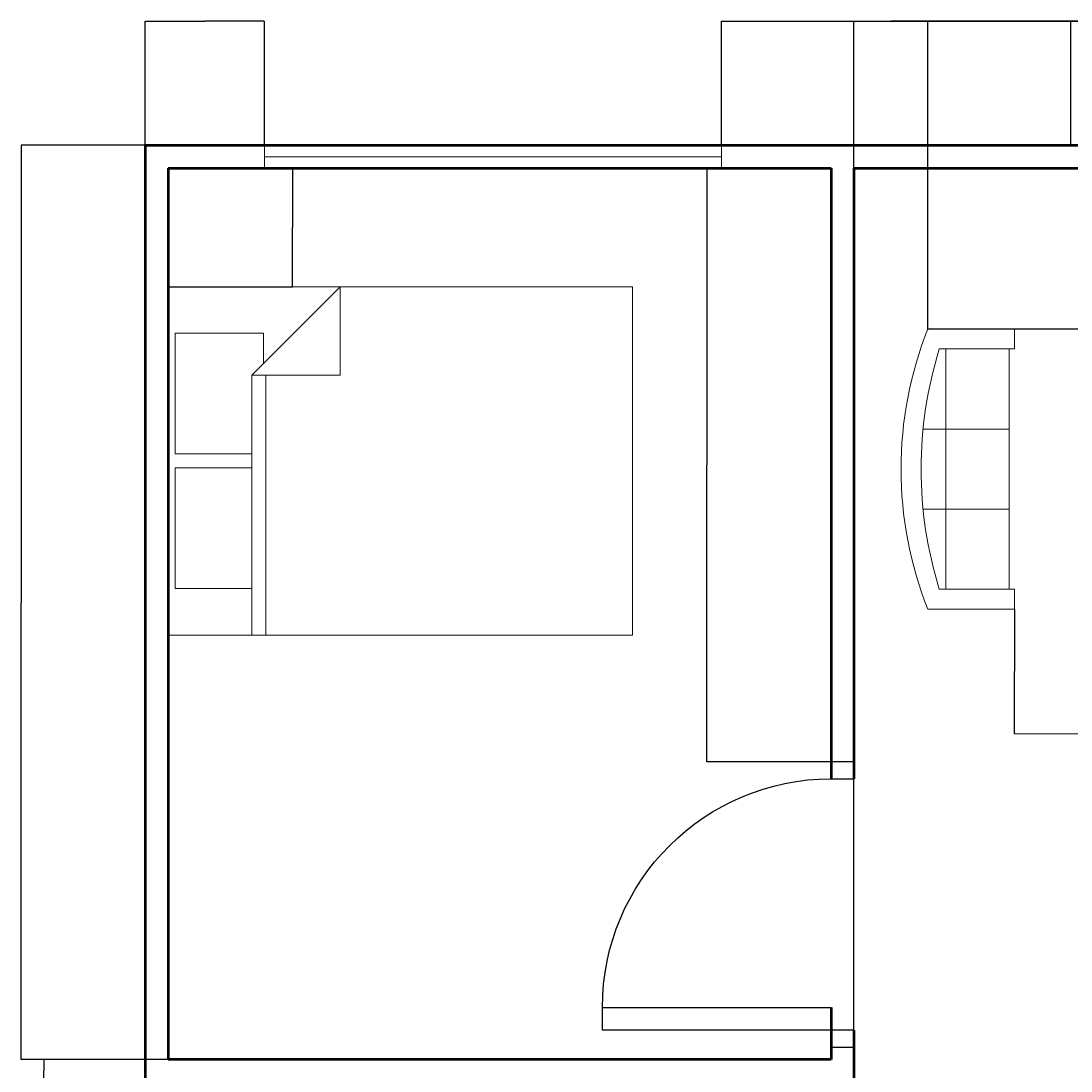
# Model space of a CAD drawing. Units: millimetres. Extents: x 1584 to 12772, y -932 to 10602.
# Tile 4 of 4: x 1584 to 6178, y 5860 to 10454. Entities that reach past the tile are written whole.
import ezdxf

# ---------------------------------------------------------------- set-up
doc = ezdxf.new("R2010")
doc.units = ezdxf.units.MM
for name, color, linetype, lineweight in [('A-ANNO-DIMS', 2, 'Continuous', 18), ('A-DOOR', 3, 'Continuous', 25), ('A-FURN', 8, 'Continuous', 18), ('A-GLAZ', 4, 'Continuous', 18), ('A-WALL', 7, 'Continuous', 50)]:
    doc.layers.add(name, color=color, linetype=linetype, lineweight=lineweight)
doc.styles.get("Standard").update_dxf_attribs({"font": 'arial.ttf'})
doc.dimstyles.get("Standard").update_dxf_attribs({"dimtxt": 0.18, "dimasz": 0.18, "dimexe": 0.18, "dimexo": 0.0625, "dimgap": 0.09, "dimtad": 0, "dimtih": 1, "dimtoh": 1, "dimdec": 4, "dimzin": 0, "dimdsep": 46, "dimtxsty": 'Standard', "dimcen": 0.09, "dimadec": 0, "dimazin": 0, "dimtfac": 1, "dimtdec": 4, "dimtofl": 0, "dimtmove": 0, "dimatfit": 3, "dimfxl": 1, "dimtolj": 1, "dimtzin": 0, "dimarcsym": 0})

# ---------------------------------------------------------------- blocks, each defined once
blk = doc.blocks.new('Bed - Queen')
for p, q in [((0, -80.00003000000002), (0, 0)), ((0, 0), (59.99998999999999, 0)), ((59.99998999999999, 0), (59.99998999999999, -80.00003000000002)), ((7.99999, -1.200000000000017), (28.79998, -1.200000000000017)), ((7.99999, -14.4), (7.99999, -1.200000000000017)), ((28.79998, -1.200000000000017), (28.79998, -14.4)), ((31.19999, -1.200000000000017), (51.99999000000001, -1.200000000000017)), ((31.19999, -14.4), (31.19999, -1.200000000000017)), ((51.99999000000001, -1.200000000000017), (51.99999000000001, -16.4)), ((0, -14.4), (44.79999999999999, -14.4)), ((59.99998999999999, -29.60000000000001), (44.79999999999999, -14.4)), ((44.79999999999999, -14.4), (44.79999999999999, -29.60000000000001)), ((44.79999999999999, -16.80000000000001), (0, -16.80000000000001)), ((51.99999000000001, -16.4), (46.79936, -16.4)), ((44.79999999999999, -29.60000000000001), (59.99998999999999, -29.60000000000001)), ((59.99998999999999, -80.00003000000002), (0, -80.00003000000002))]:
    blk.add_line(p, q)
blk = doc.blocks.new('Sofa - Roundback 7 ft.')
for p, q in [((-12.00002, -32.44210000000393), (-12.00003, -6.597100000003898)), ((11.99996999999999, -32.44210000000393), (11.99997999999999, -6.597100000003898)), ((-36.000027, -34.00000000000395), (-36.000027, -11.46960000000396)), ((35.99997999999999, -34.00000000000395), (35.99997999999999, -11.46960000000396)), ((-35.999844, -13.38190000000397), (35.99979999999999, -13.38190000000397)), ((-36.000027, -32.44210000000393), (35.99997999999999, -32.44210000000393))]:
    blk.add_line(p, q)
for points in [[(-36.000027, -34.00000000000395), (-42.000027, -34.00000000000395), (-42.000027, -8.000000000003944)], [(41.99997999999999, -8.000000000003944), (41.99997999999999, -34.00000000000395), (35.99997999999999, -34.00000000000395)]]:
    blk.add_lwpolyline(points)
for centre, radius, start, end in [((0, -114.2500000000039), 114.2500000000039, 68.43141000000072, 111.5686000000006), ((-1.00000000032e-05, -127.1968000000039), 121.1967999999973, 72.72032999999948, 107.2797000000005)]:
    blk.add_arc(centre, radius, start, end)
blk = doc.blocks.new('DOOR-SINGLE-1000')
for p, q in [((1000.000230036349, 1174.20008536707), (1000.000230036349, 1248.400085367071)), ((1000.000230036349, 1248.400085367071), (1100.000230036349, 1248.400085367071)), ((1100.000230036349, 1248.400085367071), (1100.000230036349, 1174.20008536707)), ((1000.000230036349, 1174.20008536707), (0.0002300363494214, 1174.20008536707)), ((0.0002300363494214, 1174.20008536707), (0.0002300363494214, 1074.200085367071)), ((1000.000230036349, 1074.200085367071), (1000.000230036349, 1174.20008536707)), ((1100.000230036349, 1174.20008536707), (1000.000230036349, 1174.20008536707)), ((0.0002300363494214, 1074.200085367071), (1000.000230036349, 1074.200085367071)), ((1000.000230036349, 8.53670690049e-05), (1000.000230036349, 74.20008536706973)), ((1000.000230036349, 74.20008536706973), (1100.000230036349, 74.20008536706973)), ((1100.000230036349, 74.20008536706973), (1100.000230036349, 8.53670690049e-05)), ((1100.000230036349, 8.53670690049e-05), (1000.000230036349, 8.53670690049e-05))]:
    blk.add_line(p, q)
blk.add_arc((1000.000230036349, 1074.200085367071), 1000.000000000001, 180, 270)
blk = doc.blocks.new('WIN-2000')
for p, q in [((-0.0004293290949136, 99.99960647437545), (1999.999570670905, 99.99960647437545)), ((-0.0004293290949136, -0.0003935256245313), (-0.0004293290949136, 99.99960647437545)), ((1999.999570670905, 99.99960647437545), (1999.999570670905, -0.0003935256245313)), ((-0.0004293290949136, 49.99960647437365), (1999.999570670905, 49.99960647437183)), ((1999.999570670905, -0.0003935256245313), (-0.0004293290949136, -0.0003935256245313))]:
    blk.add_line(p, q)
blk = doc.blocks.new('*D39')
at = {"layer": 'A-ANNO-DIMS', "color": 0, "lineweight": -2, "transparency": 16777216}
for p, q in [((2127.770730000001, 9910.180606000004), (1583.953230000001, 9910.180606000004)), ((1584.133230000001, 9910.000606000003), (1584.133230000001, 7910.362509137792)), ((1584.133230000002, 5910.360606000001), (1584.133230000001, 7909.998702862212)), ((2227.770730000001, 5910.180606000001), (1583.953230000002, 5910.180606))]:
    blk.add_line(p, q, dxfattribs=at)
at = {"layer": 'A-ANNO-DIMS', "color": 0, "transparency": 16777216}
for points in [[(1584.103230000001, 9910.000606000003), (1584.163230000001, 9910.000606000003), (1584.133230000001, 9910.180606000004)], [(1584.103230000002, 5910.360606000001), (1584.163230000002, 5910.360606000001), (1584.133230000002, 5910.180606)]]:
    blk.add_solid(points, dxfattribs=at)
at = {"layer": 'Defpoints', "color": 0, "transparency": 16777216}
for p in [(1584.133230000001, 9910.180606000004), (2127.833230000002, 9910.180606000004), (2227.833230000001, 5910.180606000001)]:
    blk.add_point(p, dxfattribs=at)
at = {"layer": 'A-ANNO-DIMS', "color": 0, "transparency": 16777216, "insert": (1584.133230000003, 7910.180606000001), "char_height": 0.18, "attachment_point": 5}
blk.add_mtext('\\A1;4000', dxfattribs=at)
blk = doc.blocks.new('*D40')
at = {"layer": 'A-ANNO-DIMS', "color": 0, "lineweight": -2, "transparency": 16777216}
for p, q in [((2227.770730000001, 5910.180606000001), (1683.953230000002, 5910.180606)), ((1684.133230000002, 5910.000606), (1684.133230000002, 5860.36250913779)), ((1684.133230000002, 5810.360606000001), (1684.133230000002, 5859.998702862211)), ((2227.770730000001, 5810.180606000002), (1683.953230000002, 5810.180606000001))]:
    blk.add_line(p, q, dxfattribs=at)
at = {"layer": 'A-ANNO-DIMS', "color": 0, "transparency": 16777216}
for points in [[(1684.103230000001, 5910.000606), (1684.163230000002, 5910.000606), (1684.133230000002, 5910.180606)], [(1684.103230000001, 5810.360606000001), (1684.163230000002, 5810.360606000001), (1684.133230000002, 5810.180606000001)]]:
    blk.add_solid(points, dxfattribs=at)
at = {"layer": 'Defpoints', "color": 0, "transparency": 16777216}
for p in [(1684.133230000002, 5910.180606), (2227.833230000001, 5910.180606000001), (2227.833230000001, 5810.180606000002)]:
    blk.add_point(p, dxfattribs=at)
at = {"layer": 'A-ANNO-DIMS', "color": 0, "transparency": 16777216, "insert": (1684.133230000003, 5860.180606), "char_height": 0.18, "attachment_point": 5}
blk.add_mtext('\\A1;100', dxfattribs=at)
blk = doc.blocks.new('*D44')
at = {"layer": 'A-ANNO-DIMS', "color": 0, "lineweight": -2, "transparency": 16777216}
for p, q in [((5227.83323, 312.424388), (5227.833230000001, 10454.060606)), ((5228.013230000001, 10453.880606), (7177.474826180082, 10453.880606)), ((9127.65323, 10453.880606), (7178.191633819918, 10453.880606)), ((9127.83323, 312.424388), (9127.83323, 10454.060606))]:
    blk.add_line(p, q, dxfattribs=at)
at = {"layer": 'A-ANNO-DIMS', "color": 0, "transparency": 16777216}
for points in [[(5228.013230000001, 10453.910606), (5228.013230000001, 10453.850606), (5227.833230000001, 10453.880606)], [(9127.65323, 10453.910606), (9127.65323, 10453.850606), (9127.83323, 10453.880606)]]:
    blk.add_solid(points, dxfattribs=at)
at = {"layer": 'Defpoints', "color": 0, "transparency": 16777216}
for p in [(9127.83323, 10453.880606), (5227.83323, 312.361888), (9127.83323, 312.361888)]:
    blk.add_point(p, dxfattribs=at)
at = {"layer": 'A-ANNO-DIMS', "color": 0, "transparency": 16777216, "insert": (7177.83323, 10453.880606), "char_height": 0.18, "attachment_point": 5}
blk.add_mtext('\\A1;3900', dxfattribs=at)
blk = doc.blocks.new('*D51')
at = {"layer": 'A-ANNO-DIMS', "color": 0, "lineweight": -2, "transparency": 16777216}
for p, q in [((2127.83323, 9910.243106000002), (2127.83323, 10454.060606)), ((2128.01323, 10453.880606), (2387.785711043656, 10453.880606)), ((2648.3456, 10453.880606), (2388.573118956344, 10453.880606)), ((2648.5256, 9910.243106000002), (2648.5256, 10454.060606))]:
    blk.add_line(p, q, dxfattribs=at)
at = {"layer": 'A-ANNO-DIMS', "color": 0, "transparency": 16777216}
for points in [[(2128.01323, 10453.910606), (2128.01323, 10453.850606), (2127.83323, 10453.880606)], [(2648.3456, 10453.910606), (2648.3456, 10453.850606), (2648.5256, 10453.880606)]]:
    blk.add_solid(points, dxfattribs=at)
at = {"layer": 'Defpoints', "color": 0, "transparency": 16777216}
for p in [(2648.5256, 10453.880606), (2127.83323, 9910.180606), (2648.5256, 9910.180606)]:
    blk.add_point(p, dxfattribs=at)
at = {"layer": 'A-ANNO-DIMS', "color": 0, "transparency": 16777216, "insert": (2388.179415, 10453.880606), "char_height": 0.18, "attachment_point": 5}
blk.add_mtext('\\A1;520.7', dxfattribs=at)
blk = doc.blocks.new('*D52')
at = {"layer": 'A-ANNO-DIMS', "color": 0, "lineweight": -2, "transparency": 16777216}
for p, q in [((4648.5256, 9910.243106000002), (4648.5256, 10454.060606)), ((4648.7056, 10453.880606), (5412.698189610504, 10453.880606)), ((6177.601092999999, 10453.880606), (5413.608503389494, 10453.880606)), ((6177.781093, 9910.243106000002), (6177.781093, 10454.060606))]:
    blk.add_line(p, q, dxfattribs=at)
at = {"layer": 'A-ANNO-DIMS', "color": 0, "transparency": 16777216}
for points in [[(4648.7056, 10453.910606), (4648.7056, 10453.850606), (4648.5256, 10453.880606)], [(6177.601092999999, 10453.910606), (6177.601092999999, 10453.850606), (6177.781093, 10453.880606)]]:
    blk.add_solid(points, dxfattribs=at)
at = {"layer": 'Defpoints', "color": 0, "transparency": 16777216}
for p in [(6177.781093, 10453.880606), (4648.5256, 9910.180606), (6177.781093, 9910.180606)]:
    blk.add_point(p, dxfattribs=at)
at = {"layer": 'A-ANNO-DIMS', "color": 0, "transparency": 16777216, "insert": (5413.153346499999, 10453.880606), "char_height": 0.18, "attachment_point": 5}
blk.add_mtext('\\A1;1529.3', dxfattribs=at)
blk = doc.blocks.new('*D56')
at = {"layer": 'A-ANNO-DIMS', "color": 0, "lineweight": -2, "transparency": 16777216}
for p, q in [((5127.770730000002, 9810.180606000004), (4583.953230000004, 9810.180606000004)), ((4584.133230000004, 9810.000606000003), (4584.133230000004, 8511.628021637793)), ((4584.133230000004, 7212.891631000004), (4584.133230000004, 8511.264215362215)), ((5127.770730000002, 7212.711631000003), (4583.953230000004, 7212.711631000003))]:
    blk.add_line(p, q, dxfattribs=at)
at = {"layer": 'A-ANNO-DIMS', "color": 0, "transparency": 16777216}
for points in [[(4584.103230000004, 9810.000606000003), (4584.163230000004, 9810.000606000003), (4584.133230000004, 9810.180606000004)], [(4584.103230000004, 7212.891631000004), (4584.163230000004, 7212.891631000004), (4584.133230000004, 7212.711631000003)]]:
    blk.add_solid(points, dxfattribs=at)
at = {"layer": 'Defpoints', "color": 0, "transparency": 16777216}
for p in [(4584.133230000004, 9810.180606000004), (5127.833230000002, 9810.180606000004), (5127.833230000002, 7212.711631000003)]:
    blk.add_point(p, dxfattribs=at)
at = {"layer": 'A-ANNO-DIMS', "color": 0, "transparency": 16777216, "insert": (4584.133230000006, 8511.4461185), "char_height": 0.18, "attachment_point": 5}
blk.add_mtext('\\A1;2597.5', dxfattribs=at)
blk = doc.blocks.new('*D65')
at = {"layer": 'A-ANNO-DIMS', "color": 0, "lineweight": -2, "transparency": 16777216}
for p, q in [((2227.895730000001, 9810.180606000004), (2771.713230000002, 9810.180606000004)), ((2771.533230000002, 9810.000606000003), (2771.533230000002, 9550.917519637793)), ((2771.533230000002, 9291.470627000004), (2771.533230000002, 9550.553713362217)), ((2227.895730000001, 9291.290627000002), (2771.713230000002, 9291.290627000002))]:
    blk.add_line(p, q, dxfattribs=at)
at = {"layer": 'A-ANNO-DIMS', "color": 0, "transparency": 16777216}
for points in [[(2771.503230000002, 9810.000606000003), (2771.563230000002, 9810.000606000003), (2771.533230000002, 9810.180606000004)], [(2771.503230000002, 9291.470627000004), (2771.563230000002, 9291.470627000004), (2771.533230000002, 9291.290627000002)]]:
    blk.add_solid(points, dxfattribs=at)
at = {"layer": 'Defpoints', "color": 0, "transparency": 16777216}
for p in [(2227.833230000001, 9810.180606000004), (2227.833230000001, 9291.290627000002), (2771.533230000002, 9291.290627000002)]:
    blk.add_point(p, dxfattribs=at)
at = {"layer": 'A-ANNO-DIMS', "color": 0, "transparency": 16777216, "insert": (2771.533230000005, 9550.735616500002), "char_height": 0.18, "attachment_point": 5}
blk.add_mtext('\\A1;518.9', dxfattribs=at)
blk = doc.blocks.new('*D72')
at = {"layer": 'A-ANNO-DIMS', "color": 0, "lineweight": -2, "transparency": 16777216}
for p, q in [((5227.83323, 4478.976585), (5227.83323, 10454.060606)), ((5228.013230000001, 10453.880606), (6008.25544143588, 10453.880606)), ((6789.408335, 10453.880606), (6009.166123564121, 10453.880606)), ((6789.588335000001, 4491.747446999999), (6789.588335000001, 10454.060606))]:
    blk.add_line(p, q, dxfattribs=at)
at = {"layer": 'A-ANNO-DIMS', "color": 0, "transparency": 16777216}
for points in [[(5228.013230000001, 10453.910606), (5228.013230000001, 10453.850606), (5227.83323, 10453.880606)], [(6789.408335, 10453.910606), (6789.408335, 10453.850606), (6789.588335000001, 10453.880606)]]:
    blk.add_solid(points, dxfattribs=at)
at = {"layer": 'Defpoints', "color": 0, "transparency": 16777216}
for p in [(6789.588335000001, 10453.880606), (5227.83323, 4478.914085), (6789.588335000001, 4491.684946999999)]:
    blk.add_point(p, dxfattribs=at)
at = {"layer": 'A-ANNO-DIMS', "color": 0, "transparency": 16777216, "insert": (6008.7107825, 10453.880606), "char_height": 0.18, "attachment_point": 5}
blk.add_mtext('\\A1;1561.8', dxfattribs=at)
blk = doc.blocks.new('*D74')
at = {"layer": 'A-ANNO-DIMS', "color": 0, "lineweight": -2, "transparency": 16777216}
for p, q in [((5930.629051045201, 7880.354388236549), (5929.1328585744, 7336.538946787445)), ((7586.377744045201, 7875.798948236547), (7584.881551573826, 7331.9835065789)), ((5929.313353122965, 7336.718450876363), (6756.552359239816, 7334.442478775962)), ((7584.702047484907, 7332.164001127465), (6757.463041368056, 7334.439973227866))]:
    blk.add_line(p, q, dxfattribs=at)
at = {"layer": 'A-ANNO-DIMS', "color": 0, "transparency": 16777216}
for points in [[(5929.313435661269, 7336.748450762819), (5929.31327058466, 7336.688450989905), (5929.133353804224, 7336.718946106187)], [(7584.702130023211, 7332.194001013923), (7584.701964946603, 7332.134001241009), (7584.882046803651, 7332.163505897641)]]:
    blk.add_solid(points, dxfattribs=at)
at = {"layer": 'Defpoints', "color": 0, "transparency": 16777216}
for p in [(5930.629223000001, 7880.416888), (7586.377916000002, 7875.861447999999), (5929.133353804224, 7336.718946106187)]:
    blk.add_point(p, dxfattribs=at)
at = {"layer": 'A-ANNO-DIMS', "color": 0, "transparency": 16777216, "insert": (6757.007700303936, 7334.441226001914), "char_height": 0.18, "attachment_point": 5}
blk.add_mtext('\\A1;1655.8', dxfattribs=at)
blk = doc.blocks.new('*D75')
at = {"layer": 'A-ANNO-DIMS', "color": 0, "lineweight": -2, "transparency": 16777216}
for p, q in [((5227.895730000002, 9810.180606000004), (12771.71323000001, 9810.180606000005)), ((12771.53323000001, 9810.000606000007), (12771.53323000001, 9458.68676102934)), ((12771.53323000001, 9107.008987000005), (12771.53323000001, 9458.322831970676)), ((5551.087991000002, 9106.828987000004), (12771.71323000001, 9106.828987000004))]:
    blk.add_line(p, q, dxfattribs=at)
at = {"layer": 'A-ANNO-DIMS', "color": 0, "transparency": 16777216}
for points in [[(12771.50323000001, 9810.000606000007), (12771.56323000001, 9810.000606000007), (12771.53323000001, 9810.180606000005)], [(12771.50323000001, 9107.008987000005), (12771.56323000001, 9107.008987000005), (12771.53323000001, 9106.828987000004)]]:
    blk.add_solid(points, dxfattribs=at)
at = {"layer": 'Defpoints', "color": 0, "transparency": 16777216}
for p in [(5227.833230000002, 9810.180606000004), (5551.025491000002, 9106.828987000004), (12771.53323000001, 9106.828987000004)]:
    blk.add_point(p, dxfattribs=at)
at = {"layer": 'A-ANNO-DIMS', "color": 0, "transparency": 16777216, "insert": (12771.53323000001, 9458.504796500001), "char_height": 0.18, "attachment_point": 5}
blk.add_mtext('\\A1;703.4', dxfattribs=at)
blk = doc.blocks.new('*D76')
at = {"layer": 'A-ANNO-DIMS', "color": 0, "lineweight": -2, "transparency": 16777216}
for p, q in [((5227.83323, 9810.243106000002), (5227.83323, 10454.060606)), ((5228.013230000001, 10453.880606), (5389.036638808322, 10453.880606)), ((5550.845491, 10453.880606), (5389.822082191678, 10453.880606)), ((5551.025491, 9106.891487000003), (5551.025491, 10454.060606))]:
    blk.add_line(p, q, dxfattribs=at)
at = {"layer": 'A-ANNO-DIMS', "color": 0, "transparency": 16777216}
for points in [[(5228.013230000001, 10453.910606), (5228.013230000001, 10453.850606), (5227.83323, 10453.880606)], [(5550.845491, 10453.910606), (5550.845491, 10453.850606), (5551.025491, 10453.880606)]]:
    blk.add_solid(points, dxfattribs=at)
at = {"layer": 'Defpoints', "color": 0, "transparency": 16777216}
for p in [(5551.025491, 10453.880606), (5227.83323, 9810.180606000002), (5551.025491, 9106.828987)]:
    blk.add_point(p, dxfattribs=at)
at = {"layer": 'A-ANNO-DIMS', "color": 0, "transparency": 16777216, "insert": (5389.4293605, 10453.880606), "char_height": 0.18, "attachment_point": 5}
blk.add_mtext('\\A1;323.2', dxfattribs=at)

msp = doc.modelspace()

# ---------------------------------------------------------------- linework, layer by layer
at = {"layer": 'A-GLAZ'}
for p, q in [((2648.525600213994, 9860.180606474376), (4648.525600213994, 9860.18060647438)), ((4648.525600213994, 9860.18060647438), (2648.525600213994, 9860.180606474376))]:
    msp.add_line(p, q, dxfattribs=at)
at = {"layer": 'A-WALL'}
for p, q in [((2127.833230036349, 9910.180606474376), (12227.83323003635, 9910.180606474376)), ((2127.833230036349, 9910.180606474376), (2127.833230036349, 810.1806064743769)), ((2227.833230036349, 9810.180606474374), (2227.833230036349, 5910.180606474376)), ((2227.833230036349, 9810.180606474374), (5127.833230036349, 9810.18060647438)), ((5127.833230036349, 9810.180606474374), (5127.833230036349, 7138.511630995255)), ((5227.833230036349, 9810.180606474374), (5227.83323003635, 7138.511630995253)), ((5227.833230036349, 9810.18060647438), (9127.833230036353, 9810.18060647438)), ((5127.833230036349, 6138.511630995253), (5127.833230036349, 5910.180606474376)), ((5227.83323003635, 6038.511630995254), (5227.833230036349, 5910.180606474376)), ((5127.833230036349, 5910.180606474376), (2227.833230036349, 5910.180606474376)), ((5227.833230036349, 5910.180606474376), (5227.83323003635, 5810.180606474376))]:
    msp.add_line(p, q, dxfattribs=at)

# ---------------------------------------------------------------- block references
at = {"layer": 'A-DOOR', "extrusion": (0, 0, -1), "zscale": -1, "rotation": 180}
msp.add_blockref('DOOR-SINGLE-1000', (-4127.833000000001, 7212.711716362325), dxfattribs=at)
at = {"layer": 'A-FURN', "rotation": 90}
for name, p, xscale, yscale, zscale in [('Bed - Queen', (2227.833230036349, 7767.290880652542), 25.4, 25.4, 25.4), ('Sofa - Roundback 7 ft.', (5434.224422939094, 8493.623212488268), 14.60014119084165, 14.60014119084165, 14.60014119084165)]:
    msp.add_blockref(name, p, dxfattribs=dict(at, xscale=xscale, yscale=yscale, zscale=zscale))
at = {"layer": 'A-GLAZ'}
msp.add_blockref('WIN-2000', (2648.526029543089, 9810.181), dxfattribs=at)

# ---------------------------------------------------------------- dimensions: what is measured, and where the dimension line sits
at = {"layer": 'A-ANNO-DIMS'}
for base, p1, p2, override, picture, middle in [((2648.5256, 10453.880606), (2127.83323, 9910.180606), (2648.5256, 9910.180606), {"dimdec": 1, "dimlfac": 1, "dimrnd": 0, "dimzin": 0, "dimdsep": 46, "dimlunit": 2}, '*D51', (2388.179415, 10453.880606)), ((6177.781093, 10453.880606), (4648.5256, 9910.180606), (6177.781093, 9910.180606), {"dimdec": 1, "dimlfac": 1, "dimrnd": 0, "dimzin": 0, "dimdsep": 46, "dimlunit": 2}, '*D52', (5413.153346499999, 10453.880606)), ((9127.83323, 10453.880606), (5227.83323, 312.361888), (9127.83323, 312.361888), {"dimdec": 0, "dimlfac": 1, "dimrnd": 0, "dimzin": 0, "dimdsep": 46, "dimlunit": 2}, '*D44', (7177.83323, 10453.880606)), ((6789.588335000001, 10453.880606), (5227.83323, 4478.914085), (6789.588335000001, 4491.684946999999), {"dimdec": 1, "dimlfac": 1, "dimrnd": 0, "dimzin": 0, "dimdsep": 46, "dimlunit": 2}, '*D72', (6008.7107825, 10453.880606)), ((5551.025491, 10453.880606), (5227.83323, 9810.180606000002), (5551.025491, 9106.828987), {"dimdec": 1, "dimlfac": 1, "dimrnd": 0, "dimzin": 0, "dimdsep": 46, "dimlunit": 2}, '*D76', (5389.4293605, 10453.880606))]:
    dim = msp.add_linear_dim(base=base, p1=p1, p2=p2, dimstyle='Standard', override=override, dxfattribs=at)
    dim.commit()
    dim.dimension.update_dxf_attribs({"geometry": picture, "text_midpoint": middle})
for base, p1, p2, angle, override, picture, middle in [((1584.133230000001, 9910.180606000004), (2227.83323, 5910.180606), (2127.83323, 9910.180606), 90, {"dimdec": 0, "dimlfac": 1, "dimrnd": 0, "dimzin": 0, "dimdsep": 46, "dimlunit": 2}, '*D39', (1584.133230000003, 7910.180606000001)), ((2771.533230000002, 9291.290627000002), (2227.83323, 9810.180606000002), (2227.83323, 9291.290627), 270, {"dimdec": 1, "dimlfac": 1, "dimrnd": 0, "dimzin": 0, "dimdsep": 46, "dimlunit": 2}, '*D65', (2771.533230000005, 9550.735616500002)), ((4584.133230000004, 9810.180606000004), (5127.83323, 7212.711631000001), (5127.83323, 9810.180606000002), 90.00000000000006, {"dimdec": 1, "dimlfac": 1, "dimrnd": 0, "dimzin": 0, "dimdsep": 46, "dimlunit": 2}, '*D56', (4584.133230000006, 8511.4461185)), ((12771.53323000001, 9106.828987000004), (5227.83323, 9810.180606000002), (5551.025491, 9106.828987), 90, {"dimdec": 1, "dimlfac": 1, "dimrnd": 0, "dimzin": 0, "dimdsep": 46, "dimlunit": 2}, '*D75', (12771.53323000001, 9458.504796500001)), ((5929.133353804224, 7336.718946106187), (7586.377916, 7875.861447999999), (5930.629223, 7880.416888), 179.8423632521602, {"dimdec": 1, "dimlfac": 1, "dimrnd": 0, "dimzin": 0, "dimdsep": 46, "dimlunit": 2}, '*D74', (6757.007700303936, 7334.441226001914)), ((1684.133230000002, 5910.180606), (2227.83323, 5810.180606), (2227.83323, 5910.180606), 89.99999999999947, {"dimdec": 0, "dimlfac": 1, "dimrnd": 0, "dimzin": 0, "dimdsep": 46, "dimlunit": 2}, '*D40', (1684.133230000003, 5860.180606))]:
    dim = msp.add_linear_dim(base=base, p1=p1, p2=p2, angle=angle, dimstyle='Standard', override=override, dxfattribs=at)
    dim.commit()
    dim.dimension.update_dxf_attribs({"geometry": picture, "text_midpoint": middle})

doc.saveas('drawing.dxf')
